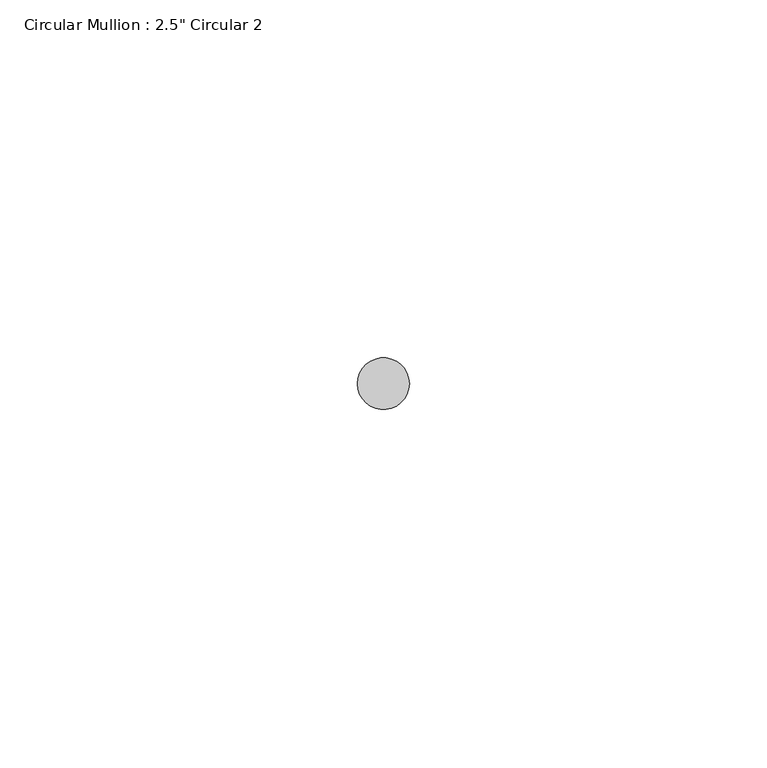
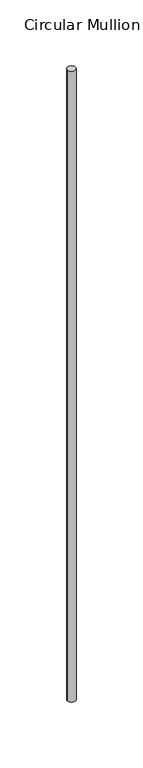
"""IFC4 building model written with IfcOpenShell, lengths in millimetres: member geometry."""

from ifc_helpers import new_model, si_unit, point, frame, frame_2d, origin, place, context, project, spatial, circle_curve, trimmed, segment, composite_curve, outline, extrude, source, transform, mapped, element, save


def member_02ee8d56(model_context):
    return source(origin(), model_context, "Body", "SweptSolid", [
        extrude(outline(composite_curve([segment(trimmed(circle_curve(frame_2d((-3.6195, 0.0)), 3.6195), [point((0.0, 0.0))], [point((-7.239, 0.0))], False, "CARTESIAN"), True, "CONTINUOUS"), segment(trimmed(circle_curve(frame_2d((-3.6195, 0.0)), 3.6195), [point((-7.239, 0.0))], [point((0.0, 0.0))], False, "CARTESIAN"), True, "CONTINUOUS")], self_intersect=False)), frame((0.0, 0.0, -592.6666667), z_axis=(0.0, 0.0, 1.0), x_axis=(1.0, 0.0, 0.0)), (0.0, 0.0, 1.0), 592.6666667),
    ])


if __name__ == "__main__":
    model = new_model("IFC4")
    model_context = context("Model", 3, world=origin())
    ifc_project = project(units=[si_unit("LENGTHUNIT", "METRE", prefix="MILLI")], contexts=[model_context])
    site = spatial("IfcSite", under=ifc_project)
    building = spatial("IfcBuilding", under=site)
    placement = place(None, origin())
    member_shape = member_02ee8d56(model_context)
    element("IfcMember", 1, ObjectType="Circular Mullion : 2.5\" Circular 2", at=placement, inside=building, context=model_context, shape_type="MappedRepresentation", body=[
        mapped(member_shape, transform((0.0, 0.0, 0.0), x_axis=(1.0, 0.0, 0.0), y_axis=(0.0, 1.0, 0.0), z_axis=(0.0, 0.0, 1.0))),
    ])
    save(model, "model.ifc")

# Revit data of these elements
# Type "Circular Mullion : 2.5\" Circular 2"
#   built-in parameter 1007350 = 0.011875 (stored number, unit not read)
# Element 1 (IfcMember, "Circular Mullion : 2.5\" Circular 2")
#   Materials on its faces: "Aluminum"
# Materials
#   "Aluminum": class "Metal", colour RGB 247 247 247, transparency 0, Description = "Aluminum 6061", Cost = 0
